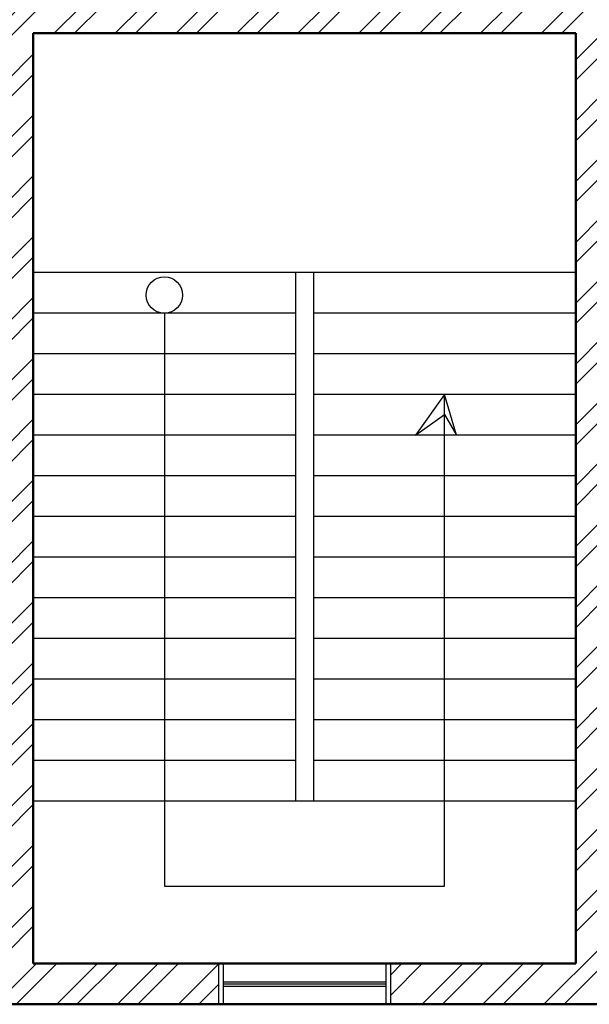
# Model space of a CAD drawing. Units: inches. Extents: x -31485 to -28799, y 18003 to 19130.
# Tile 2 of 15: x -30999 to -30873, y 18180 to 18398. Entities that reach past the tile are written whole.
import ezdxf

# ---------------------------------------------------------------- set-up
doc = ezdxf.new("R2010")
doc.units = ezdxf.units.IN
for name, color, linetype, lineweight in [('A-FLOR-STRS', 3, 'Continuous', 25), ('A-GLAZ', 4, 'Continuous', 25), ('A-WALL', 7, 'Continuous', 50), ('A-WALL-PATT', 8, 'Continuous', 13)]:
    doc.layers.add(name, color=color, linetype=linetype, lineweight=lineweight)

# ---------------------------------------------------------------- blocks, each defined once
blk = doc.blocks.new('WIN-900-W9')
for p, q in [((-29982.20533134393, 18824.1159329289), (-29982.20533134393, 18815.1159329289)), ((-29981.20533134393, 18824.1159329289), (-29981.20533134393, 18815.1159329289)), ((-29945.20533134393, 18824.1159329289), (-29945.20533134393, 18815.1159329289)), ((-29944.20533134393, 18824.1159329289), (-29944.20533134393, 18815.1159329289)), ((-29981.20533134393, 18820.1159329289), (-29945.20533134393, 18820.1159329289)), ((-29981.20533134393, 18819.6159329289), (-29945.20533134393, 18819.6159329289)), ((-29981.20533134393, 18819.1159329289), (-29945.20533134393, 18819.1159329289))]:
    blk.add_line(p, q)

msp = doc.modelspace()

# ---------------------------------------------------------------- hatches: boundary and pattern name
at = {"layer": 'A-WALL-PATT'}
h = msp.add_hatch(dxfattribs=at)
h.set_pattern_fill('ANSI32', color=256)
h.set_pattern_definition([(45, (-1687.357050595019, -0.3129728357926069), (-6.735192090801865, 6.735192090801866), []), (45, (-1682.866920595021, -0.3129728357926069), (-6.735192090801865, 6.735192090801866), [])])
h.paths.add_polyline_path([(-31156.52828769349, 18823.80296009311), (-31209.52828769349, 18823.80296009311), (-31209.52828769349, 18761.80296009311), (-31200.52828769349, 18761.80296009311), (-31200.52828769349, 18814.80296009311), (-31156.52828769349, 18814.80296009311)], flags=17)
h.paths.add_polyline_path([(-31022.5282876935, 18823.80296009311), (-31118.52828769349, 18823.80296009311), (-31118.52828769349, 18814.80296009311), (-31074.52828769349, 18814.80296009311), (-31074.52828769349, 18720.78574754094), (-31070.95696393926, 18720.78574754094), (-31068.52828769349, 18720.75952290947), (-31068.52828769349, 18814.80296009311), (-31022.5282876935, 18814.80296009311)], flags=17)
h.paths.add_polyline_path([(-30754.52828769349, 18823.80296009311), (-30850.5282876935, 18823.80296009311), (-30850.5282876935, 18814.80296009311), (-30806.5282876935, 18814.80296009311), (-30806.52828769349, 18723.10029278397), (-30800.5282876935, 18723.10029278397), (-30800.5282876935, 18814.80296009311), (-30754.52828769349, 18814.80296009311)], flags=17)
h.paths.add_polyline_path([(-30661.52828769349, 18823.80296009311), (-30716.52828769349, 18823.80296009311), (-30716.52828769349, 18814.80296009311), (-30670.52828769349, 18814.80296009311), (-30670.52828769349, 18761.80296009311), (-30661.52828769349, 18761.80296009311)], flags=17)
h.paths.add_polyline_path([(-30986.91891278487, 18670.80296009311), (-31068.52828769349, 18670.80296009311), (-31068.52828769349, 18684.75952290947), (-31074.52828769349, 18684.75952290947), (-31074.52828769349, 18670.80296009311), (-31200.52828769349, 18670.80296009311), (-31200.52828769349, 18723.80296009311), (-31209.52828769349, 18723.80296009311), (-31209.52828769349, 18641.80296009311), (-31200.52828769349, 18641.80296009311), (-31200.52828769349, 18664.80296009311), (-31104.52828769349, 18664.80296009311), (-31104.52828769349, 18628.92834044014), (-31098.52828769349, 18628.92834044014), (-31098.52828769348, 18664.8029600931), (-30986.91891278488, 18664.8029600931)], flags=17)
h.paths.add_polyline_path([(-30661.52828769349, 18723.80296009311), (-30670.52828769349, 18723.80296009311), (-30670.52828769349, 18670.80296009311), (-30800.5282876935, 18670.80296009311), (-30800.5282876935, 18687.10029278396), (-30806.52828769349, 18687.10029278396), (-30806.52828769349, 18670.80296009311), (-30885.59628027248, 18670.80296009311), (-30885.59628027248, 18667.80293426455), (-30885.59628027248, 18664.80296009311), (-30760.52828769349, 18664.80296009311), (-30760.52828769349, 18625.80296009311), (-30754.52828769349, 18625.80296009311), (-30754.52828769349, 18664.80296009311), (-30670.52828769349, 18664.80296009311), (-30670.52828769349, 18641.80296009311), (-30661.52828769349, 18641.80296009311)], flags=17)
h.paths.add_polyline_path([(-31200.52828769349, 18574.80296009311), (-31188.56436894977, 18574.80296009311), (-31188.56436894977, 18580.80296009311), (-31200.52828769349, 18580.80296009311), (-31200.52828769349, 18603.80296009311), (-31209.52828769349, 18603.80296009311), (-31209.52828769349, 18557.80296009311), (-31200.52828769349, 18557.80296009311)], flags=17)
h.paths.add_polyline_path([(-31098.52828769349, 18592.92834044014), (-31104.52828769349, 18592.92834044014), (-31104.52828769349, 18580.80296009311), (-31164.56436894977, 18580.80296009311), (-31164.56436894977, 18574.80296009311), (-31104.52828769349, 18574.80296009311), (-31104.52828769349, 18514.80296009311), (-31200.52828769349, 18514.80296009311), (-31200.52828769349, 18531.80296009311), (-31209.52828769349, 18531.80296009311), (-31209.52828769349, 18473.80296009311), (-31200.52828769349, 18473.80296009311), (-31200.52828769349, 18508.80296009311), (-31056.52828769349, 18508.80296009312), (-31056.52828769349, 18501.62307445529), (-31050.52828769349, 18501.62307445529), (-31050.52828769349, 18514.80296009311), (-31098.52828769349, 18514.80296009311)], flags=17)
h.paths.add_polyline_path([(-30661.52828769349, 18531.80296009311), (-30670.52828769349, 18531.80296009311), (-30670.52828769349, 18514.80296009311), (-30754.52828769349, 18514.80296009311), (-30754.52828769349, 18574.80296009311), (-30700.74522746605, 18574.80296009311), (-30700.74522746605, 18577.44024221289), (-30700.74522746605, 18580.8029600931), (-30754.52828769349, 18580.80296009311), (-30754.52828769349, 18589.80296009311), (-30760.52828769349, 18589.80296009311), (-30760.52828769349, 18514.80296009311), (-30820.52828769349, 18514.80296009311), (-30820.52828769348, 18499.26438911774), (-30814.52828769349, 18499.26438911774), (-30814.52828769349, 18508.80296009311), (-30670.52828769349, 18508.80296009311), (-30670.52828769349, 18473.80296009311), (-30661.52828769349, 18473.80296009311)], flags=17)
h.paths.add_polyline_path([(-30661.52828769349, 18435.80296009311), (-30670.52828769349, 18435.80296009311), (-30670.52828769349, 18400.80296009311), (-30814.52828769349, 18400.80296009311), (-30814.52828769349, 18413.15176302367), (-30820.52828769349, 18413.15176302367), (-30820.52828769349, 18400.80296009311), (-30932.52828769349, 18400.80296009311), (-30932.52828769349, 18664.80296009311), (-30921.59628027248, 18664.80296009311), (-30921.59628027248, 18670.80296009311), (-30932.5282876935, 18670.80296009311), (-30932.5282876935, 18814.80296009311), (-30888.5282876935, 18814.80296009311), (-30888.5282876935, 18823.80296009311), (-30984.5282876935, 18823.80296009311), (-30984.5282876935, 18814.80296009311), (-30938.5282876935, 18814.80296009311), (-30938.5282876935, 18670.80296009311), (-30950.91891278487, 18670.80296009311), (-30950.91891278488, 18664.80296009311), (-30938.5282876935, 18664.80296009311), (-30938.52828769349, 18400.80296009311), (-31050.52828769349, 18400.80296009311), (-31050.52828769349, 18411.18080736427), (-31056.52828769348, 18411.18080736427), (-31056.52828769348, 18400.80296009311), (-31200.52828769349, 18400.80296009311), (-31200.52828769349, 18435.80296009311), (-31209.52828769349, 18435.80296009311), (-31209.52828769349, 18179.80296009311), (-31200.52828769349, 18179.80296009311), (-31200.52828769349, 18394.80296009311), (-31001.52828769348, 18394.80296009311), (-31001.52828769348, 18179.80296009311), (-30954.52828769347, 18179.80296009311), (-30954.52828769347, 18188.80296009311), (-30995.52828769348, 18188.80296009311), (-30995.52828769348, 18394.80296009311), (-30875.52828769348, 18394.80296009311), (-30875.52828769348, 18188.80296009311), (-30916.52828769347, 18188.80296009311), (-30916.52828769347, 18179.80296009311), (-30869.52828769348, 18179.80296009311), (-30869.52828769348, 18394.80296009311), (-30670.52828769349, 18394.80296009311), (-30670.52828769349, 18179.80296009311), (-30661.52828769349, 18179.80296009311)])

# ---------------------------------------------------------------- linework, layer by layer
at = {"layer": 'A-FLOR-STRS'}
for p, q in [((-30875.52828769347, 18341.80296009311), (-30995.52828769348, 18341.80296009311)), ((-30937.52828769349, 18341.80296009311), (-30937.52828769349, 18224.80296009311)), ((-30933.52828769348, 18341.80296009311), (-30933.52828769349, 18224.80296009311)), ((-30937.52828769349, 18332.80296009311), (-30995.52828769348, 18332.80296009311)), ((-30966.52828769349, 18332.80296009311), (-30966.52828769349, 18205.95510239493)), ((-30875.52828769347, 18332.80296009311), (-30933.52828769349, 18332.80296009311)), ((-30937.52828769349, 18323.80296009311), (-30995.52828769348, 18323.80296009311)), ((-30875.52828769347, 18323.80296009311), (-30933.52828769349, 18323.80296009311)), ((-30937.52828769349, 18314.80296009311), (-30995.52828769348, 18314.80296009311)), ((-30875.52828769347, 18314.80296009311), (-30933.52828769349, 18314.80296009311)), ((-30904.52828769346, 18314.80296009311), (-30910.98467026646, 18305.80296009311)), ((-30904.52828769347, 18205.95510239493), (-30904.52828769346, 18314.80296009311)), ((-30901.87148909437, 18305.80296009311), (-30904.52828769346, 18314.80296009311)), ((-30910.98467026646, 18305.80296009311), (-30904.52828769346, 18310.3547463713)), ((-30904.52828769346, 18310.3547463713), (-30901.87148909437, 18305.80296009311)), ((-30937.52828769349, 18305.80296009311), (-30995.52828769348, 18305.80296009311)), ((-30875.52828769347, 18305.80296009311), (-30933.52828769349, 18305.80296009311)), ((-30937.52828769349, 18296.80296009311), (-30995.52828769348, 18296.80296009311)), ((-30875.52828769347, 18296.80296009311), (-30933.52828769349, 18296.80296009311)), ((-30937.52828769349, 18287.80296009311), (-30995.52828769348, 18287.80296009311)), ((-30875.52828769347, 18287.80296009311), (-30933.52828769349, 18287.80296009311)), ((-30937.52828769349, 18278.80296009311), (-30995.52828769348, 18278.80296009311)), ((-30875.52828769347, 18278.80296009311), (-30933.52828769349, 18278.80296009311)), ((-30937.52828769349, 18269.80296009311), (-30995.52828769348, 18269.80296009311)), ((-30875.52828769347, 18269.80296009311), (-30933.52828769349, 18269.80296009311)), ((-30937.52828769349, 18260.80296009311), (-30995.52828769348, 18260.80296009311)), ((-30875.52828769347, 18260.80296009311), (-30933.52828769349, 18260.80296009311)), ((-30937.52828769349, 18251.80296009311), (-30995.52828769348, 18251.80296009311)), ((-30875.52828769347, 18251.80296009311), (-30933.52828769349, 18251.80296009311)), ((-30937.52828769349, 18242.80296009311), (-30995.52828769348, 18242.80296009311)), ((-30875.52828769347, 18242.80296009311), (-30933.52828769349, 18242.80296009311)), ((-30937.52828769349, 18233.80296009311), (-30995.52828769348, 18233.80296009311)), ((-30875.52828769347, 18233.80296009311), (-30933.52828769349, 18233.80296009311)), ((-30875.52828769347, 18224.80296009311), (-30995.52828769348, 18224.80296009311)), ((-30966.52828769349, 18205.95510239493), (-30904.52828769347, 18205.95510239493))]:
    msp.add_line(p, q, dxfattribs=at)
msp.add_circle((-30966.52828769349, 18336.83946940413), 4.036509311019472, dxfattribs=at)
at = {"layer": 'A-WALL'}
for p, q in [((-30995.52828769348, 18394.80296009311), (-30875.52828769349, 18394.80296009311)), ((-30995.52828769348, 18394.80296009311), (-30995.52828769348, 18188.80296009311)), ((-30875.52828769348, 18394.80296009311), (-30875.52828769348, 18188.80296009311)), ((-30875.52828769347, 18188.80296009311), (-30995.52828769348, 18188.80296009311)), ((-30869.52828769348, 18179.80296009311), (-31001.52828769348, 18179.80296009311))]:
    msp.add_line(p, q, dxfattribs=at)

# ---------------------------------------------------------------- block references
at = {"layer": 'A-GLAZ'}
msp.add_blockref('WIN-900-W9', (-972.3229563445057, -635.3129728277854), dxfattribs=at)

doc.saveas('drawing.dxf')
